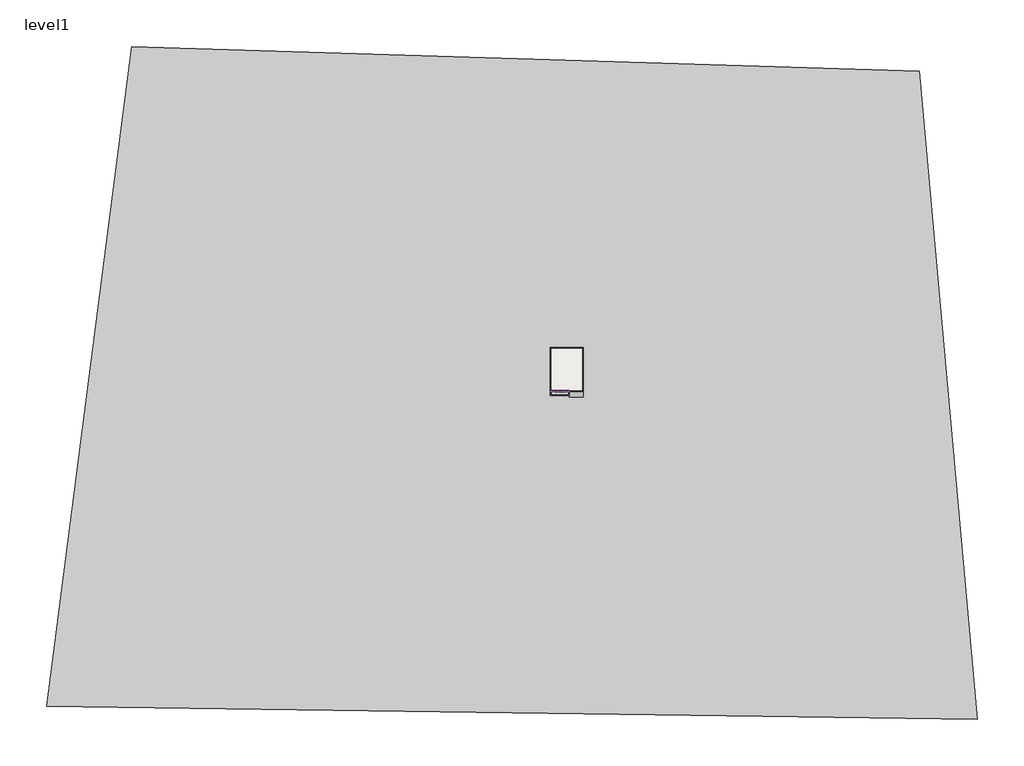
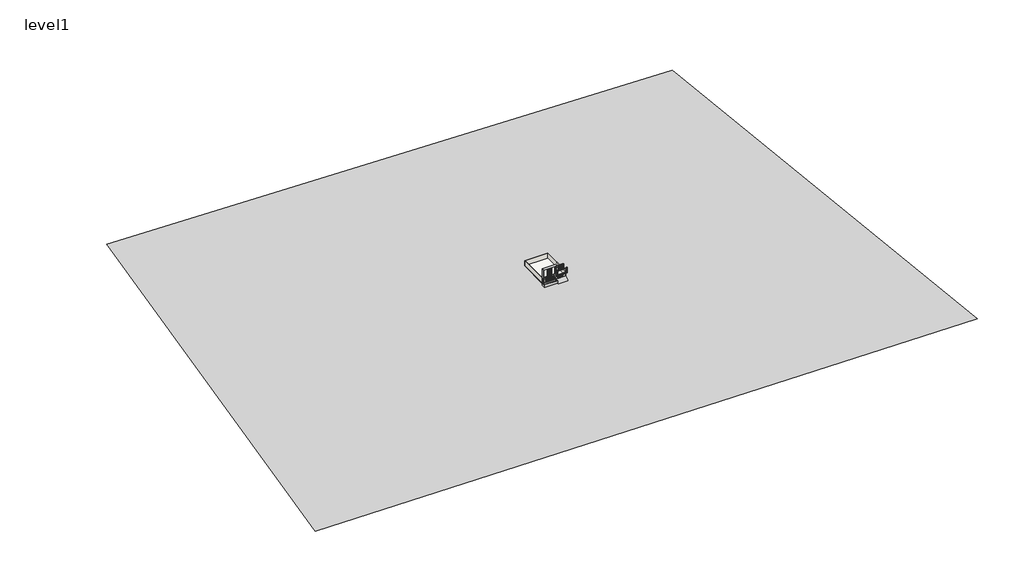
# One storey: 6 walls, 2 dampers, 1 door, 1 duct fitting, 1 proxy, 1 slab.
"""IFC4 building model written with IfcOpenShell, lengths in millimetres."""

from ifc_helpers import new_model, si_unit, frame, origin, place, context, project, spatial, polyline, outline, extrude, faceted_brep, triangles, transform, mapped, element, save
from components import duct_accessories_1_duct_accessories_1_02249294, duct_accessories_2_duct_accessories_2_621c73fd, door_97be9440, duct_fittings_1_duct_fittings_1_d2289eb8

model = new_model("IFC4")

# Units and contexts
model_context = context("Model", 3, world=origin())
ifc_project = project(units=[si_unit("LENGTHUNIT", "METRE", prefix="MILLI")], contexts=[model_context])

# Site, building, storey
site = spatial("IfcSite", under=ifc_project)
building = spatial("IfcBuilding", under=site)
storey = spatial("IfcBuildingStorey", under=building, Name="level1", Elevation=3000.0)

# Proxy
placement = place(None, origin())
element("IfcBuildingElementProxy", 1, Name="Building Element Proxy", at=placement, inside=storey, context=model_context, shape_type="Tessellation", body=[
    triangles([(-129437.7178711, 92105.6895996, 1894.3518127), (92188.6147705, 85090.3317627, 1894.3518127), (108611.156543, -97444.8427734, 1894.3518127), (-153494.147168, -93740.8456055, 1894.3518127)], [[1, 4, 2], [3, 2, 4]], closed=False),
])

# Dampers
duct_accessories_1_duct_accessories_1_shape = duct_accessories_1_duct_accessories_1_02249294(model_context)
element("IfcDamper", 2, ObjectType="Duct Accessories 1 : Duct Accessories 1", at=placement, inside=storey, context=model_context, shape_type="MappedRepresentation", body=[
    mapped(duct_accessories_1_duct_accessories_1_shape, transform((0.0, 0.0, 0.0), x_axis=(1.0, 0.0, 0.0), y_axis=(0.0, 1.0, 0.0), z_axis=(0.0, 0.0, 1.0))),
])
duct_accessories_2_duct_accessories_2_shape = duct_accessories_2_duct_accessories_2_621c73fd(model_context)
element("IfcDamper", 3, ObjectType="Duct Accessories 2 : Duct Accessories 2", at=placement, inside=storey, context=model_context, shape_type="MappedRepresentation", body=[
    mapped(duct_accessories_2_duct_accessories_2_shape, transform((0.0, 0.0, 0.0), x_axis=(1.0, 0.0, 0.0), y_axis=(0.0, 1.0, 0.0), z_axis=(0.0, 0.0, 1.0))),
])

# Door
door_shape = door_97be9440(model_context)
element("IfcDoor", 4, at=placement, inside=storey, context=model_context, shape_type="MappedRepresentation", body=[
    mapped(door_shape, transform((-4618.8043842, -4990.9296146, 3000.0), x_axis=(1.0, 0.0, 0.0), y_axis=(0.0, 1.0, 0.0), z_axis=(0.0, 0.0, 1.0))),
])

# Duct fitting
duct_fittings_1_duct_fittings_1_shape = duct_fittings_1_duct_fittings_1_d2289eb8(model_context)
element("IfcDuctFitting", 5, ObjectType="Duct Fittings 1 : Duct Fittings 1", at=placement, inside=storey, context=model_context, shape_type="MappedRepresentation", body=[
    mapped(duct_fittings_1_duct_fittings_1_shape, transform((0.0, 0.0, 0.0), x_axis=(1.0, 0.0, 0.0), y_axis=(0.0, 1.0, 0.0), z_axis=(0.0, 0.0, 1.0))),
])

# Slab
element("IfcSlab", 6, ObjectType="Generic 150mm", at=placement, inside=storey, context=model_context, shape_type="SweptSolid", body=[
    extrude(outline(polyline([(-2353.4667042, 7341.0703854), (-2353.4667042, -4990.9296146), (-11637.4667042, -4990.9296146), (-11637.4667042, 7341.0703854), (-2353.4667042, 7341.0703854)])), frame((0.0, 0.0, 2850.0), z_axis=(0.0, 0.0, 1.0), x_axis=(1.0, 0.0, 0.0)), (0.0, 0.0, 1.0), 150.0),
])

# Walls
element("IfcWall", 7, ObjectType="Generic - 140mm Masonry", at=placement, inside=storey, context=model_context, shape_type="Brep", body=[
    faceted_brep([(-11637.4667042, -4990.9296146, 3000.0), (-6315.8667042, -4990.9296146, 3000.0), (-6315.8667042, -4990.9296146, 5000.0), (-11637.4667042, -4990.9296146, 5000.0), (-11637.4667042, -4850.9296146, 3000.0), (-11637.4667042, -4850.9296146, 5000.0), (-11497.4667042, -4850.9296146, 5000.0), (-6315.8667042, -4850.9296146, 5000.0), (-6315.8667042, -4850.9296146, 3000.0), (-11497.4667042, -4850.9296146, 3000.0), (-6315.8667042, -4920.9296146, 3000.0)], [[[0, 1, 2, 3]], [[4, 5, 6, 7, 8, 9]], [[1, 0, 4, 9, 8, 10]], [[2, 1, 10, 8, 7]], [[3, 2, 7, 6, 5]], [[0, 3, 5, 4]]]),
])
element("IfcWall", 8, ObjectType="Generic - 140mm Masonry", at=placement, inside=storey, context=model_context, shape_type="Brep", body=[
    faceted_brep([(-2353.4667042, -5060.9296146, 3000.0), (-2353.4667042, 7341.0703854, 3000.0), (-2353.4667042, 7341.0703854, 5000.0), (-2353.4667042, -5060.9296146, 5000.0), (-2493.4667042, -5060.9296146, 3000.0), (-2493.4667042, -5060.9296146, 3813.3686956), (-2493.4667042, -5060.9296146, 5000.0), (-2493.4667042, 7201.0703854, 5000.0), (-2493.4667042, 7341.0703854, 5000.0), (-2493.4667042, 7341.0703854, 3000.0), (-2493.4667042, 7201.0703854, 3000.0), (-2493.4667042, -4920.9296146, 3000.0)], [[[0, 1, 2, 3]], [[4, 5, 6, 7, 8, 9, 10, 11]], [[1, 0, 4, 11, 10, 9]], [[3, 2, 8, 7, 6]], [[2, 1, 9, 8]], [[0, 3, 6, 5, 4]]]),
])
element("IfcWall", 9, ObjectType="Generic - 140mm Masonry", at=placement, inside=storey, context=model_context, shape_type="Brep", body=[
    faceted_brep([(-2493.4667042, 7341.0703854, 3000.0), (-11637.4667042, 7341.0703854, 3000.0), (-11637.4667042, 7341.0703854, 5000.0), (-2493.4667042, 7341.0703854, 5000.0), (-2493.4667042, 7201.0703854, 3000.0), (-2493.4667042, 7201.0703854, 5000.0), (-11497.4667042, 7201.0703854, 5000.0), (-11637.4667042, 7201.0703854, 5000.0), (-11637.4667042, 7201.0703854, 3000.0), (-11497.4667042, 7201.0703854, 3000.0)], [[[0, 1, 2, 3]], [[4, 5, 6, 7, 8, 9]], [[1, 0, 4, 9, 8]], [[3, 2, 7, 6, 5]], [[0, 3, 5, 4]], [[2, 1, 8, 7]]]),
])
element("IfcWall", 10, ObjectType="Generic - 140mm Masonry", at=placement, inside=storey, context=model_context, shape_type="SweptSolid", body=[
    extrude(outline(polyline([(-11637.4667042, -4850.9296146), (-11637.4667042, 7201.0703854), (-11497.4667042, 7201.0703854), (-11497.4667042, -4850.9296146), (-11637.4667042, -4850.9296146)])), frame((0.0, 0.0, 3000.0), z_axis=(0.0, 0.0, 1.0), x_axis=(1.0, 0.0, 0.0)), (0.0, 0.0, 1.0), 2000.0),
])
element("IfcWall", 11, ObjectType="Generic - 140mm Masonry", at=placement, inside=storey, context=model_context, shape_type="SweptSolid", body=[
    extrude(outline(polyline([(-2493.4667042, -4920.9296146), (-2493.4667042, -5060.9296146), (-3575.8043842, -5060.9296146), (-3575.8043842, -4963.4631031), (-3609.8043842, -4963.4631031), (-3609.8043842, -4920.9296146), (-2493.4667042, -4920.9296146)])), frame((0.0, 0.0, 3000.0), z_axis=(0.0, 0.0, 1.0), x_axis=(1.0, 0.0, 0.0)), (0.0, 0.0, 1.0), 813.3686956),
])
element("IfcWall", 12, ObjectType="Generic - 140mm Masonry", at=placement, inside=storey, context=model_context, shape_type="Brep", body=[
    faceted_brep([(-6315.8667042, -5060.9296146, 3000.0), (-5634.8043842, -5060.9296146, 3000.0), (-5634.8043842, -5060.9296146, 3813.3686956), (-6315.8667042, -5060.9296146, 3813.3686956), (-6315.8667042, -4920.9296146, 3000.0), (-6315.8667042, -4920.9296146, 3813.3686956), (-5634.8043842, -4920.9296146, 3813.3686956), (-5634.8043842, -4920.9296146, 3000.0), (-6315.8667042, -4990.9296146, 3000.0)], [[[0, 1, 2, 3]], [[4, 5, 6, 7]], [[1, 0, 8, 4, 7]], [[2, 1, 7, 6]], [[3, 2, 6, 5]], [[0, 3, 5, 4, 8]]]),
])

save(model, "model.ifc")

# Revit data of these elements
# Type
#   Type Mark = "40"
#   Version Revit = "Revit 2017"
#   Uniformat II description = "Double door"
#   Uniformat CSI = "B2030"
#   URL = "https://www.fenetremeo.com/porte-entree"
#   Type de pose = "Tunnel"
#   Référence modèle = "MeO-PE-BALADE-2vtx"
#   Pose vitrage = "Vitrage collé"
#   Keynote = "MeO-PE-BALADE-2vtx"
#   Neuf / Réno = "Rénovation"
#   Model = "Porte double BALADE"
#   Matériaux = "Aluminium / bois"
#   IFC version = "IFC 2x3 Coordination 2.0"
#   IFC classification = "Door"
#   Fiches produits = "https://www.fenetremeo.com/porte-entree"
#   Famille de produit = "Porte"
#   Manufacturer = "MéO"
#   FILE_NAME = "2021-07-MeO-PE-BALADE-2vtx"
#   Design = "Modélisation non contractuelle"
#   Description = "Porte 2 vantaux égaux"
#   Contraintes largeur porte = "700 < Largeur < 1200"
#   Contraintes hauteur porte = "1953 < Hauteur < 2500"
#   Contraintes hauteur poignée porte = "900 <Hauteur poignée < 1300"
#   Analytic Construction = "<Aucun>"
#   Coefficient thermique Ud = "0.72 / 0.75 Ud"
#   BIMobject main category = "Exterior carpentry"
#   Avis technique = "https://www.fcba.fr/wp-content/uploads/2020/10/rc_nf297.pdf"
#   Surface = 7854.671916 ft
#   Pose tunnel = 0.032808 ft
#   Longueur de traverse haute 33,43,53,63,73,83 = 0.108268 ft
#   Largeur zone 2 = 3.28084 ft
#   Largeur zone 1 = 3.28084 ft
#   Largeur du dormant 33,43,53,63,73,83 = 0.108268 ft
#   Rough Width = 6.843832 ft
#   Hauteur poignée = 3.608924 ft
#   Hauteur dormant = 4 ft
#   Rough Height = 4 ft
#   HT ouvrant = 3.826115 ft
#   Height = 3.888451 ft
#   Width = 6.627297 ft
#   Doublage 75,105,125,145,165,185,205 = 0.286964 ft
#   Message Hors abaques = yes
#   Hors abaques = yes
#   Vitrage = Verre
#   Couleur poignée = Acier inoxydable AISI 304
#   Choix du modèle = element 399773
#   Function = (empty or 0)
#   Wall Closure = (empty or 0)
# Type "Generic 150mm"
#   Function = 0
#   Layers, outside or top first: 0.492126 ft no material (function 1)
# Type "Generic - 140mm Masonry"
#   Layers, outside or top first: 0.459318 ft "Concrete Masonry Units" (function 1)
# Element 1 (IfcBuildingElementProxy)
#   Material = Default New Material
#   Phase Created = New Construction
# Element 2 (IfcDamper, "Duct Accessories 1 : Duct Accessories 1")
#   Mark = "1"
#   Phase Created = New Construction
#   Materials on its faces: "Clad - White", "Wood - Stained"
# Element 3 (IfcDamper, "Duct Accessories 2 : Duct Accessories 2")
#   Mark = "2"
#   Phase Created = New Construction
#   Materials on its faces: "GREY"
# Element 4 (IfcDoor)
#   Phase Created = New Construction
#   Materials on its faces: "Acier inoxydable AISI 304", "Verre", "Aluminium"
# Element 5 (IfcDuctFitting, "Duct Fittings 1 : Duct Fittings 1")
#   Phase Created = New Construction
#   Materials on its faces: "RC"
# Element 6 (IfcSlab, "Generic 150mm")
#   Height Offset From Level = 0 ft
#   Phase Created = New Construction
#   Materials on its faces: "Default Floor"
# Element 7 (IfcWall, "Generic - 140mm Masonry")
#   Top Offset = 0 ft
#   Base Offset = 0 ft
#   wall height = 6.56168 ft
#   Phase Created = New Construction
#   Base Constraint = level1
#   Top Constraint = level 2
#   Materials on its faces: "Concrete Masonry Units", "GREY", "Cherry"
# Element 8 (IfcWall, "Generic - 140mm Masonry")
#   Top Offset = 0 ft
#   Base Offset = 0 ft
#   wall height = 6.56168 ft
#   Phase Created = New Construction
#   Base Constraint = level1
#   Top Constraint = level 2
#   Materials on its faces: "Concrete Masonry Units", "Cherry", "YELLOW", "Clad - White"
# Element 9 (IfcWall, "Generic - 140mm Masonry")
#   Top Offset = 0 ft
#   Base Offset = 0 ft
#   wall height = 6.56168 ft
#   Phase Created = New Construction
#   Base Constraint = level1
#   Top Constraint = level 2
#   Materials on its faces: "Concrete Masonry Units", "PAINT", "Cherry"
# Element 10 (IfcWall, "Generic - 140mm Masonry")
#   Top Offset = 0 ft
#   Base Offset = 0 ft
#   wall height = 6.56168 ft
#   Phase Created = New Construction
#   Base Constraint = level1
#   Top Constraint = level 2
#   Materials on its faces: "Concrete Masonry Units", "Cherry", "YELLOW"
# Elements 11, 12 (IfcWall, "Generic - 140mm Masonry")
#   built-in parameter 1001111 = 0 ft
#   Top Offset = 0 ft
#   Base Offset = 0 ft
#   Unconnected Height = 2.668532 ft
#   wall height = 2.668532 ft
#   Phase Created = New Construction
#   Base Constraint = level1
#   Materials on its faces: "Concrete Masonry Units", "Clad - White"
# Materials
#   "Verre": class "Verre", colour RGB 92 99 177, transparency 0.7, Description = "Verre sodocalcique", Cost = 0
#   "Acier inoxydable AISI 304": colour RGB 120 120 120, transparency 0, Description = "Stainless Steel 18/8", Cost = 0
#   "Concrete Masonry Units": class "Masonry", colour RGB 181 181 181, transparency 0, Description = "Concrete masonry units", Cost = 0
#   "Default New Material": class "Generic", colour RGB 40 117 68, transparency 0, Cost = 0
#   "Clad - White": class "Wood", colour RGB 242 242 238, transparency 0, Cost = 0
#   "Wood - Stained": class "Wood", colour RGB 224 178 126, transparency 0, Cost = 0
#   "GREY": class "Generic", colour RGB 176 176 176, transparency 0, Cost = 0
#   "Aluminium": class "Metal", colour RGB 247 247 247, transparency 0, Description = "Aluminium 6061", Cost = 0
#   "RC": class "Generic", colour RGB 255 255 255, transparency 0, Cost = 0
#   "Default Floor": colour RGB 127 127 127, transparency 0, Cost = 0
#   "Cherry": class "Wood", colour RGB 226 177 128, transparency 0, Description = "Prunus Serotina", Cost = 0
#   "YELLOW": class "Generic", colour RGB 255 255 0, transparency 0, Cost = 0
#   "PAINT": class "Generic", colour RGB 105 77 58, transparency 0, Cost = 0
